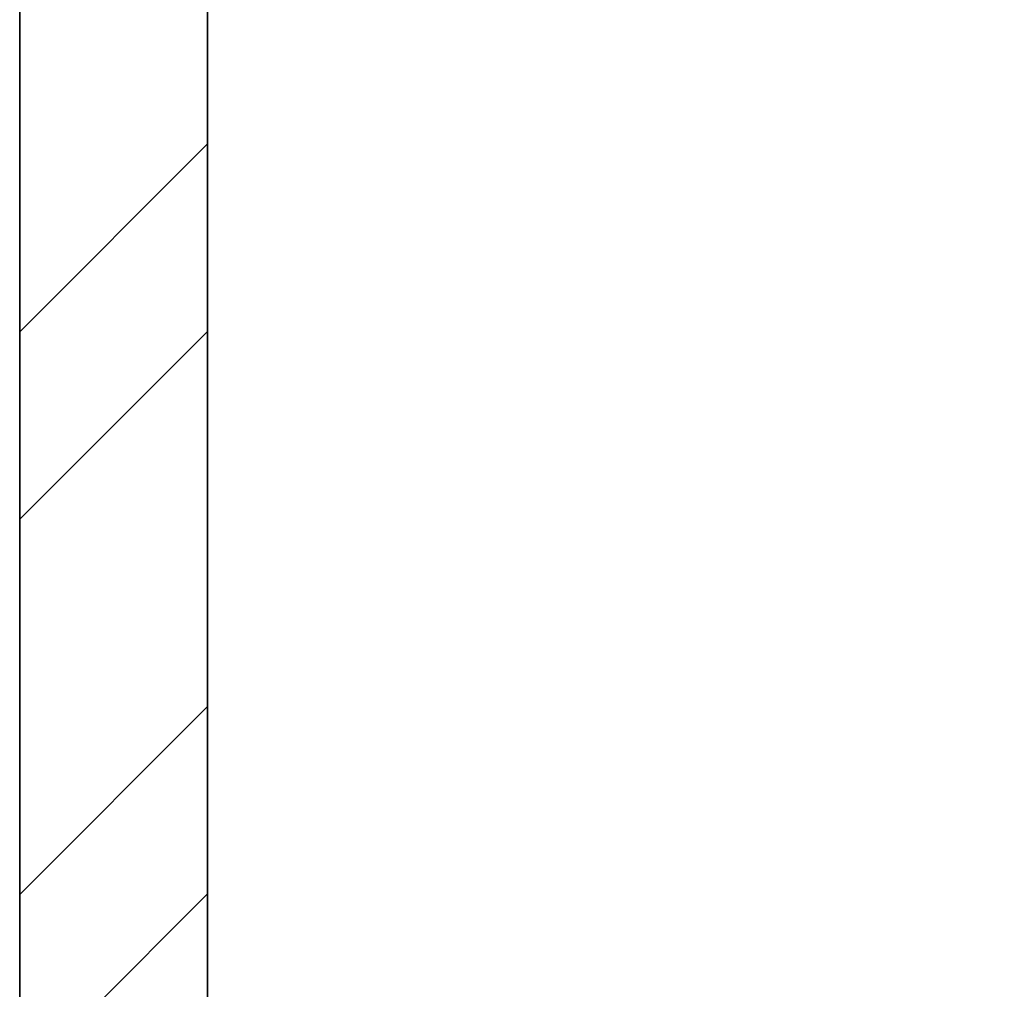
# Model space of a CAD drawing. Units: inches. Extents: x 2168 to 3056, y 1130 to 2629.
# Tile 8 of 42: x 2645 to 2669, y 1956 to 1979. Entities that reach past the tile are written whole.
import ezdxf

# ---------------------------------------------------------------- set-up
doc = ezdxf.new("R2010")
doc.units = ezdxf.units.IN
doc.layers.add('A-WALL', color=7, linetype='Continuous', lineweight=35)
doc.layers.add('A-WALL-PATT', color=143, linetype='Continuous', lineweight=13, true_color=0x7aafdf)

msp = doc.modelspace()

# ---------------------------------------------------------------- hatches: boundary and pattern name
at = {"layer": 'A-WALL-PATT'}
h = msp.add_hatch(dxfattribs=at)
h.set_pattern_fill('ANSI32', color=256)
h.paths.add_polyline_path([(2463.796, 2409.389), (2467.387, 2409.389), (2467.387, 2413.889), (2454.768, 2413.889), (2454.768, 2411.639), (2454.768, 2409.389), (2459.296, 2409.389), (2459.296, 2265.389), (2455.644, 2265.389), (2455.644, 2260.889), (2467.349, 2260.889), (2467.349, 2263.139), (2467.349, 2265.389), (2463.796, 2265.389)])
h.paths.add_polyline_path([(2431.596, 2413.889), (2409.647, 2413.889), (2409.647, 2409.389), (2431.596, 2409.389), (2431.596, 2411.639)])
h.paths.add_polyline_path([(2349.647, 2413.889), (2331.796, 2413.889), (2331.796, 2362.671), (2336.296, 2362.671), (2336.296, 2409.389), (2349.647, 2409.389), (2349.647, 2411.639)])
h.paths.add_polyline_path([(2634.149, 2411.639), (2634.149, 2413.889), (2562.293, 2413.889), (2562.293, 2409.389), (2595.796, 2409.389), (2595.796, 2280.309), (2595.826, 2280.309), (2595.826, 2265.389), (2499.91, 2265.389), (2499.91, 2260.889), (2550.796, 2260.889), (2550.796, 2117.308), (2555.296, 2117.308), (2555.296, 2168.08), (2571.93, 2168.08), (2571.93, 2176.889), (2559.796, 2176.889), (2559.796, 2256.389), (2640.796, 2256.389), (2640.796, 2176.889), (2626.428, 2176.889), (2626.428, 2168.08), (2645.296, 2168.08), (2645.296, 2116.637), (2649.796, 2116.637), (2649.796, 2260.889), (2691.251, 2260.889), (2691.251, 2263.139), (2691.251, 2265.389), (2670.655, 2265.389), (2670.655, 2265.365), (2600.296, 2265.365), (2600.296, 2280.258), (2600.296, 2409.389), (2634.149, 2409.389)])
h.paths.add_polyline_path([(2600.296, 2473.889), (2612.84, 2473.889), (2612.84, 2478.389), (2572.636, 2478.389), (2572.636, 2473.889), (2595.796, 2473.889), (2595.796, 2413.889), (2600.296, 2413.889)])
h.paths.add_polyline_path([(2535.796, 2473.889), (2548.636, 2473.889), (2548.636, 2478.389), (2531.396, 2478.389), (2531.396, 2413.889), (2521.6, 2413.889), (2521.6, 2409.389), (2539.239, 2409.389), (2539.239, 2411.639), (2539.239, 2413.889), (2535.796, 2413.889)])
h.paths.add_polyline_path([(2664.796, 2478.389), (2636.84, 2478.389), (2636.84, 2473.889), (2660.296, 2473.889), (2660.296, 2413.889), (2656.165, 2413.889), (2656.165, 2409.389), (2671.684, 2409.389), (2671.684, 2411.639), (2671.684, 2413.889), (2664.796, 2413.889)])
h.paths.add_polyline_path([(2705.942, 2413.889), (2695.684, 2413.889), (2695.684, 2409.389), (2705.942, 2409.389)])
h.paths.add_polyline_path([(2741.35, 2413.889), (2728.733, 2413.889), (2728.733, 2411.639), (2728.733, 2409.389), (2732.296, 2409.389), (2732.296, 2265.389), (2725.733, 2265.389), (2725.733, 2260.889), (2740.917, 2260.889), (2740.917, 2263.139), (2740.917, 2265.389), (2736.796, 2265.389), (2736.796, 2409.389), (2741.35, 2409.389)])
h.paths.add_polyline_path([(2785.655, 2413.889), (2764.546, 2413.889), (2764.486, 2409.389), (2785.655, 2409.389), (2785.655, 2411.639)])
h.paths.add_polyline_path([(2864.296, 2413.889), (2845.655, 2413.889), (2845.655, 2409.389), (2859.796, 2409.389), (2859.796, 2368.425), (2864.296, 2368.425)])
h.paths.add_polyline_path([(2864.296, 2308.425), (2862.046, 2308.425), (2859.796, 2308.425), (2859.796, 2265.389), (2774.483, 2265.389), (2774.483, 2263.139), (2774.483, 2260.889), (2781.796, 2260.889), (2781.796, 2226.654), (2786.296, 2226.654), (2786.296, 2260.889), (2859.796, 2260.889), (2859.796, 2241.352), (2864.296, 2241.352)])
h.paths.add_polyline_path([(2864.296, 2217.352), (2862.046, 2217.352), (2859.796, 2217.352), (2859.796, 2200.889), (2786.296, 2200.889), (2786.296, 2205.931), (2784.046, 2205.931), (2781.796, 2205.931), (2781.796, 2150.974), (2786.296, 2150.974), (2786.296, 2161.889), (2859.796, 2161.889), (2859.796, 2144.419), (2864.296, 2144.419)])
h.paths.add_polyline_path([(2859.796, 2196.389), (2859.796, 2166.389), (2786.296, 2166.389), (2786.296, 2196.389)], flags=16)
h.paths.add_polyline_path([(2864.296, 2108.419), (2862.046, 2108.419), (2859.796, 2108.419), (2859.796, 2080.889), (2786.296, 2080.889), (2786.296, 2111.993), (2781.796, 2111.993), (2781.796, 2080.889), (2649.796, 2080.889), (2649.796, 2086.036), (2647.546, 2086.036), (2645.296, 2086.036), (2645.296, 2071.739), (2649.796, 2071.739), (2649.796, 2076.389), (2781.796, 2076.389), (2781.796, 2041.792), (2786.296, 2041.792), (2786.296, 2076.389), (2859.796, 2076.389), (2859.796, 2058.577), (2864.296, 2058.577)])
h.paths.add_polyline_path([(2864.296, 2022.577), (2859.796, 2022.577), (2859.796, 1992.389), (2786.296, 1992.389), (2786.296, 1999.573), (2781.796, 1999.573), (2781.796, 1848.085), (2784.046, 1848.085), (2786.296, 1848.085), (2786.296, 1851.389), (2859.796, 1851.389), (2859.796, 1838.258), (2864.296, 1838.258)], flags=17)
h.paths.add_polyline_path([(2859.796, 1987.889), (2859.796, 1855.889), (2786.296, 1855.889), (2786.296, 1987.889)], flags=16)
h.paths.add_polyline_path([(2823.046, 1987.889), (2841.421, 1921.889), (2823.046, 1855.889)], flags=0)
h.paths.add_polyline_path([(2864.296, 1814.258), (2859.796, 1814.258), (2859.796, 1791.389), (2786.296, 1791.389), (2786.296, 1825.658), (2784.046, 1825.658), (2781.796, 1825.658), (2781.796, 1791.389), (2720.155, 1791.389), (2720.155, 1791.265), (2649.796, 1791.265), (2649.796, 1806.159), (2649.796, 2038.983), (2647.546, 2038.983), (2645.296, 2038.983), (2645.296, 1783.925), (2649.796, 1783.925), (2649.796, 1786.889), (2781.796, 1786.889), (2781.796, 1746.789), (2786.296, 1746.789), (2786.296, 1786.889), (2859.796, 1786.889), (2859.796, 1770.083), (2864.296, 1770.083)])
h.paths.add_polyline_path([(2864.296, 1734.083), (2862.046, 1734.083), (2859.796, 1734.083), (2859.796, 1705.889), (2786.296, 1705.889), (2786.296, 1714.166), (2781.796, 1714.166), (2781.796, 1660.527), (2786.296, 1660.527), (2786.296, 1666.889), (2859.796, 1666.889), (2859.796, 1648.342), (2864.296, 1648.342)])
h.paths.add_polyline_path([(2786.296, 1701.389), (2859.796, 1701.389), (2859.796, 1671.389), (2786.296, 1671.389)], flags=16)
h.paths.add_polyline_path([(2649.796, 1756.576), (2647.546, 1756.576), (2645.296, 1756.576), (2645.296, 1606.889), (2555.296, 1606.889), (2555.296, 1749.513), (2553.046, 1749.513), (2550.796, 1749.513), (2550.796, 1606.889), (2503.006, 1606.889), (2503.006, 1604.639), (2503.006, 1602.389), (2595.796, 1602.389), (2595.849, 1602.389), (2595.849, 1587.495), (2595.796, 1458.389), (2561.502, 1458.389), (2561.502, 1456.139), (2561.502, 1453.889), (2595.796, 1453.889), (2595.796, 1381.889), (2573.438, 1381.889), (2573.438, 1377.389), (2613.01, 1377.389), (2613.01, 1379.639), (2613.01, 1381.889), (2600.296, 1381.889), (2600.296, 1453.889), (2634.327, 1453.889), (2634.327, 1458.389), (2600.296, 1458.389), (2600.296, 1602.389), (2670.655, 1602.389), (2694.095, 1602.389), (2694.095, 1606.889), (2649.796, 1606.889)])
h.paths.add_polyline_path([(2736.796, 1602.389), (2741.562, 1602.389), (2741.562, 1606.889), (2726.203, 1606.889), (2726.203, 1604.639), (2726.203, 1602.389), (2732.296, 1602.389), (2732.296, 1458.389), (2727.899, 1458.389), (2727.899, 1453.889), (2740.821, 1453.889), (2740.821, 1456.139), (2740.821, 1458.389), (2736.796, 1458.389)])
h.paths.add_polyline_path([(2859.796, 1606.889), (2786.296, 1606.889), (2786.296, 1637.334), (2784.046, 1637.334), (2781.796, 1637.334), (2781.796, 1606.889), (2775.612, 1606.889), (2775.612, 1602.389), (2859.796, 1602.389)])
h.paths.add_polyline_path([(2864.296, 1624.342), (2862.046, 1624.342), (2859.796, 1624.342), (2859.796, 1570.39), (2864.296, 1570.39)])
h.paths.add_polyline_path([(2864.296, 1510.39), (2862.046, 1510.39), (2859.796, 1510.39), (2859.796, 1458.389), (2846.735, 1458.389), (2846.735, 1456.139), (2846.735, 1453.889), (2864.296, 1453.889)])
h.paths.add_polyline_path([(2786.735, 1458.389), (2765.444, 1458.389), (2765.444, 1453.889), (2786.735, 1453.889)])
h.paths.add_polyline_path([(2706.004, 1458.389), (2695.36, 1458.389), (2695.36, 1453.889), (2706.004, 1453.889), (2706.004, 1456.139)])
h.paths.add_polyline_path([(2671.36, 1456.139), (2671.36, 1458.389), (2655.986, 1458.389), (2655.986, 1456.139), (2655.986, 1453.889), (2660.296, 1453.889), (2660.296, 1381.889), (2637.01, 1381.889), (2637.01, 1377.389), (2664.796, 1377.389), (2664.796, 1453.889), (2671.36, 1453.889)], flags=17)
h.paths.add_polyline_path([(2539.829, 1458.389), (2520.237, 1458.389), (2520.237, 1453.889), (2531.296, 1453.889), (2531.296, 1377.389), (2546.449, 1377.389), (2546.449, 1379.639), (2546.449, 1381.889), (2535.796, 1381.889), (2535.796, 1453.889), (2539.829, 1453.889)], flags=17)
h.paths.add_polyline_path([(2496.237, 1458.389), (2489.13, 1458.389), (2489.13, 1453.889), (2496.237, 1453.889), (2496.237, 1456.139)])
h.paths.add_polyline_path([(2467.433, 1456.139), (2467.433, 1458.389), (2463.796, 1458.389), (2463.796, 1602.389), (2468.242, 1602.389), (2468.242, 1605.7), (2468.242, 1606.889), (2454.602, 1606.889), (2454.602, 1602.389), (2459.296, 1602.389), (2459.296, 1458.389), (2454.24, 1458.389), (2454.24, 1453.889), (2467.433, 1453.889)])
h.paths.add_polyline_path([(2431.601, 1456.139), (2431.601, 1458.389), (2411.386, 1458.389), (2411.386, 1453.889), (2431.601, 1453.889)])
h.paths.add_polyline_path([(2351.386, 1458.389), (2336.296, 1458.389), (2336.296, 1490.693), (2334.046, 1490.693), (2331.796, 1490.693), (2331.796, 1453.889), (2351.386, 1453.889), (2351.386, 1456.139)])
h.paths.add_polyline_path([(2336.296, 1629.705), (2331.796, 1629.705), (2331.796, 1552.317), (2336.296, 1552.317), (2336.296, 1602.389), (2406.655, 1602.389), (2423.472, 1602.389), (2423.472, 1606.889), (2418.796, 1606.889), (2418.796, 1643.678), (2416.546, 1643.678), (2414.296, 1643.678), (2414.296, 1606.889), (2336.296, 1606.889)])
h.paths.add_polyline_path([(2418.796, 1714.384), (2414.296, 1714.384), (2414.296, 1705.889), (2336.296, 1705.889), (2336.296, 1731.324), (2334.046, 1731.324), (2331.796, 1731.324), (2331.796, 1653.705), (2334.046, 1653.705), (2336.296, 1653.705), (2336.296, 1666.889), (2414.296, 1666.889), (2414.296, 1663.589), (2418.796, 1663.589)])
h.paths.add_polyline_path([(2336.296, 1701.389), (2414.296, 1701.389), (2414.296, 1671.389), (2336.296, 1671.389)], flags=16)
h.paths.add_polyline_path([(2555.296, 2040.059), (2550.796, 2040.059), (2550.796, 1791.389), (2550.561, 1791.205), (2480.202, 1791.205), (2418.796, 1791.389), (2418.796, 1825.448), (2416.546, 1825.448), (2414.296, 1825.448), (2414.296, 1791.389), (2336.296, 1791.389), (2336.296, 1806.409), (2331.796, 1806.409), (2331.796, 1767.324), (2336.296, 1767.324), (2336.296, 1786.889), (2414.296, 1786.889), (2414.296, 1745.457), (2418.796, 1745.457), (2418.796, 1786.889), (2550.796, 1786.889), (2550.796, 1783.011), (2555.296, 1783.011)])
h.paths.add_polyline_path([(2418.796, 1923.389), (2423.207, 1923.389), (2423.207, 1925.639), (2423.207, 1927.889), (2418.796, 1927.889), (2418.796, 2000.048), (2414.296, 2000.048), (2414.296, 1992.389), (2336.296, 1992.389), (2336.296, 1987.889), (2414.296, 1987.889), (2414.296, 1855.889), (2336.296, 1855.889), (2336.296, 1851.389), (2414.296, 1851.389), (2414.296, 1846.759), (2418.796, 1846.759)], flags=17)
h.paths.add_polyline_path([(2336.296, 2019.294), (2334.046, 2019.294), (2331.796, 2019.294), (2331.796, 1830.409), (2336.296, 1830.409)], flags=17)
h.paths.add_polyline_path([(2550.796, 1927.889), (2453.541, 1927.889), (2453.541, 1925.639), (2453.541, 1923.389), (2550.796, 1923.389)], flags=17)
h.paths.add_polyline_path([(2744.987, 1927.889), (2649.796, 1927.889), (2649.796, 1923.389), (2744.987, 1923.389), (2744.987, 1925.639)], flags=17)
h.paths.add_polyline_path([(2555.296, 2086.458), (2553.046, 2086.458), (2550.796, 2086.458), (2550.796, 2080.889), (2418.796, 2080.889), (2336.296, 2080.889), (2336.296, 2115.399), (2334.046, 2115.399), (2331.796, 2115.399), (2331.796, 2055.294), (2336.296, 2055.294), (2336.296, 2076.389), (2550.796, 2076.389), (2550.796, 2071.538), (2555.296, 2071.538)])
h.paths.add_polyline_path([(2418.796, 2121.389), (2414.296, 2121.389), (2414.296, 2080.889), (2418.796, 2080.889)])
h.paths.add_polyline_path([(2418.796, 2076.389), (2414.296, 2076.389), (2414.296, 2035.123), (2418.796, 2035.123)])
h.paths.add_polyline_path([(2422.868, 2263.139), (2422.868, 2265.389), (2406.655, 2265.389), (2406.655, 2265.359), (2336.296, 2265.359), (2336.296, 2280.252), (2336.296, 2302.671), (2334.046, 2302.671), (2331.796, 2302.671), (2331.796, 2246.853), (2336.296, 2246.853), (2336.296, 2260.889), (2414.296, 2260.889), (2414.296, 2223.996), (2418.796, 2223.996), (2418.796, 2260.889), (2422.868, 2260.889)])
h.paths.add_polyline_path([(2418.796, 2204.783), (2416.546, 2204.783), (2414.296, 2204.783), (2414.296, 2200.889), (2336.296, 2200.889), (2336.296, 2220.853), (2331.796, 2220.853), (2331.796, 2151.399), (2336.296, 2151.399), (2336.296, 2161.889), (2414.296, 2161.889), (2414.296, 2153.726), (2418.796, 2153.726)])
h.paths.add_polyline_path([(2414.296, 2196.389), (2414.296, 2166.389), (2336.296, 2166.389), (2336.296, 2196.389)], flags=16)
h.paths.add_polyline_path([(2375.296, 2181.389), (2336.296, 2166.389), (2336.296, 2196.389)], flags=0)
h.paths.add_polyline_path([(2809.595, 2172.34), (2838.804, 2172.34), (2838.804, 2190.997), (2809.595, 2190.997)], flags=8)
h.paths.add_polyline_path([(2849.75, 1919.585), (2849.75, 1952.672), (2831.093, 1952.672), (2831.093, 1919.585)], flags=8)
h.paths.add_polyline_path([(2808.875, 1901.967), (2808.875, 1937.85), (2790.149, 1937.85), (2790.149, 1901.967)], flags=8)
h.paths.add_polyline_path([(2806.285, 1671.896), (2835.493, 1671.896), (2835.493, 1690.553), (2806.285, 1690.553)], flags=8)
h.paths.add_polyline_path([(2353.186, 1676.549), (2382.395, 1676.549), (2382.395, 1695.207), (2353.186, 1695.207)], flags=8)
h.paths.add_polyline_path([(2360.083, 1832.308), (2389.241, 1832.308), (2389.241, 1850.966), (2360.083, 1850.966)], flags=25)
h.paths.add_polyline_path([(2354.822, 2167.823), (2384.031, 2167.823), (2384.031, 2186.481), (2354.822, 2186.481)], flags=8)

# ---------------------------------------------------------------- linework, layer by layer
at = {"layer": 'A-WALL'}
for p, q in [((2649.796, 1791.389), (2649.796, 2040.564)), ((2645.296, 2038.983), (2645.296, 1783.925))]:
    msp.add_line(p, q, dxfattribs=at)

doc.saveas('drawing.dxf')
